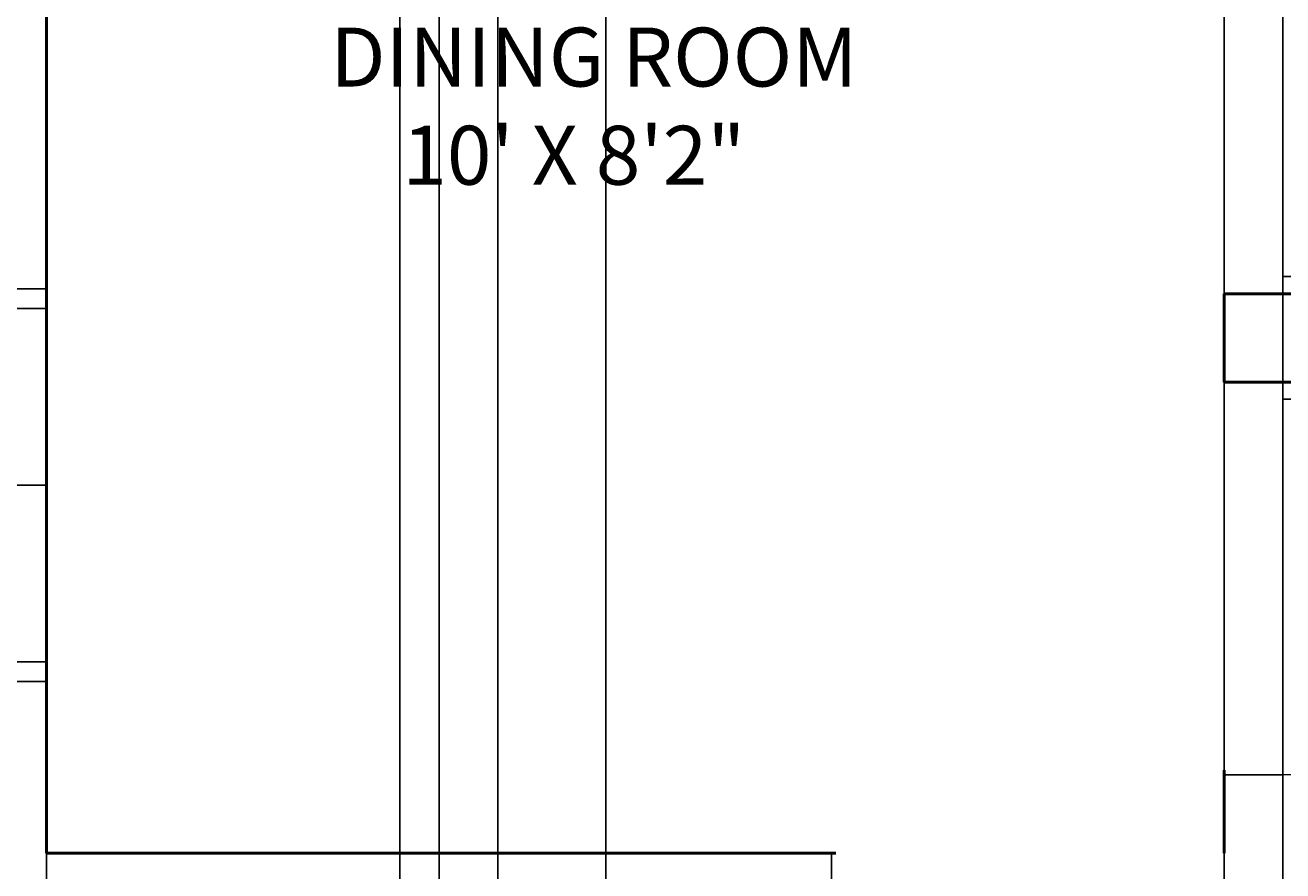
# Model space of a CAD drawing. Units: inches. Extents: x 37 to 824, y -700 to 234.
# Tile 36 of 77: x 168 to 296, y -161 to -75. Entities that reach past the tile are written whole.
import ezdxf

# ---------------------------------------------------------------- set-up
doc = ezdxf.new("R2010")
doc.units = ezdxf.units.IN
doc.header["$MEASUREMENT"] = 0
for name, color, linetype, lineweight in [('A-ANNO-DIMS', 2, 'Continuous', 18), ('A-AREA-IDEN', 3, 'Continuous', 18), ('A-DOOR', 4, 'Continuous', 25), ('A-GLAZ', 4, 'Continuous', 25), ('A-WALL', 2, 'Continuous', 50)]:
    doc.layers.add(name, color=color, linetype=linetype, lineweight=lineweight)
doc.styles.get("Standard").update_dxf_attribs({"font": 'arial.ttf'})
doc.dimstyles.get("Standard").update_dxf_attribs({"dimtxt": 0.18, "dimasz": 0.18, "dimexe": 0.18, "dimexo": 0.0625, "dimgap": 0.09, "dimtad": 0, "dimtih": 1, "dimtoh": 1, "dimdec": 1, "dimzin": 0, "dimdsep": 46, "dimlunit": 4, "dimtxsty": 'Standard', "dimcen": 0.09, "dimadec": 0, "dimazin": 0, "dimtfac": 1, "dimtdec": 1, "dimtofl": 0, "dimtmove": 0, "dimatfit": 3, "dimfxl": 1, "dimtolj": 1, "dimtzin": 0, "dimarcsym": 0})

# ---------------------------------------------------------------- blocks, each defined once
blk = doc.blocks.new('*U5')
for p, q in [((0, 0), (0, 6)), ((40, 0), (40, 6))]:
    blk.add_line(p, q)
blk.add_lwpolyline([(0, 0), (0, -40), (1.75, -40), (1.75, 0)], close=True)
blk.add_arc((0, 0), 40, 270, 0)
blk = doc.blocks.new('*U2')
for p, q in [((-40, 0), (-40, 6)), ((0, 0), (0, 6))]:
    blk.add_line(p, q)
blk.add_lwpolyline([(0, 0), (0, -40), (-1.75, -40), (-1.75, 0)], close=True)
blk.add_arc((0, 0), 40, 180, 270)
blk = doc.blocks.new('WIN-900')
for p, q in [((0, 9), (0, 0)), ((2, 9), (2, 0)), ((20, 9), (20, 0)), ((38, 9), (38, 0)), ((40, 9), (40, 0)), ((38, 5.5), (2, 5.5)), ((38, 3.5), (2, 3.5))]:
    blk.add_line(p, q)
blk = doc.blocks.new('*D77')
at = {"layer": 'A-ANNO-DIMS', "color": 0, "lineweight": -2, "ltscale": 0.5, "transparency": 16777216}
for p, q in [((227.08, 45.5), (227.08, -400.41)), ((290.08, 15.03), (290.08, -400.41)), ((227.26, -400.23), (258.25, -400.23)), ((289.9, -400.23), (258.91, -400.23))]:
    blk.add_line(p, q, dxfattribs=at)
at = {"layer": 'A-ANNO-DIMS', "color": 0, "ltscale": 0.5, "transparency": 16777216}
for points in [[(227.26, -400.2), (227.26, -400.26), (227.08, -400.23)], [(289.9, -400.2), (289.9, -400.26), (290.08, -400.23)]]:
    blk.add_solid(points, dxfattribs=at)
at = {"layer": 'Defpoints', "color": 0, "ltscale": 0.5, "transparency": 16777216}
for p in [(227.08, 45.56), (290.08, 15.09), (290.08, -400.23)]:
    blk.add_point(p, dxfattribs=at)
at = {"layer": 'A-ANNO-DIMS', "color": 0, "ltscale": 0.5, "transparency": 16777216, "insert": (258.58, -400.23), "char_height": 0.18, "attachment_point": 5}
blk.add_mtext('\\A1;5\'-3"', dxfattribs=at)
blk = doc.blocks.new('*D84')
at = {"layer": 'A-ANNO-DIMS', "color": 0, "lineweight": -2, "ltscale": 0.5, "transparency": 16777216}
for p, q in [((170.08, -265.85), (170.08, 234.17)), ((170.26, 233.99), (189.75, 233.99)), ((209.9, 233.99), (190.41, 233.99)), ((210.08, -265.85), (210.08, 234.17))]:
    blk.add_line(p, q, dxfattribs=at)
at = {"layer": 'A-ANNO-DIMS', "color": 0, "ltscale": 0.5, "transparency": 16777216}
for points in [[(170.26, 234.02), (170.26, 233.96), (170.08, 233.99)], [(209.9, 234.02), (209.9, 233.96), (210.08, 233.99)]]:
    blk.add_solid(points, dxfattribs=at)
at = {"layer": 'Defpoints', "color": 0, "ltscale": 0.5, "transparency": 16777216}
for p in [(210.08, 233.99), (170.08, -265.91), (210.08, -265.91)]:
    blk.add_point(p, dxfattribs=at)
at = {"layer": 'A-ANNO-DIMS', "color": 0, "ltscale": 0.5, "transparency": 16777216, "insert": (190.08, 233.99), "char_height": 0.18, "attachment_point": 5}
blk.add_mtext('\\A1;3\'-4"', dxfattribs=at)
blk = doc.blocks.new('*D85')
at = {"layer": 'A-ANNO-DIMS', "color": 0, "lineweight": -2, "ltscale": 0.5, "transparency": 16777216}
for p, q in [((170.08, -356.85), (170.08, 234.17)), ((170.26, 233.99), (187.75, 233.99)), ((205.9, 233.99), (188.41, 233.99)), ((206.08, -356.85), (206.08, 234.17))]:
    blk.add_line(p, q, dxfattribs=at)
at = {"layer": 'A-ANNO-DIMS', "color": 0, "ltscale": 0.5, "transparency": 16777216}
for points in [[(170.26, 234.02), (170.26, 233.96), (170.08, 233.99)], [(205.9, 234.02), (205.9, 233.96), (206.08, 233.99)]]:
    blk.add_solid(points, dxfattribs=at)
at = {"layer": 'Defpoints', "color": 0, "ltscale": 0.5, "transparency": 16777216}
for p in [(206.08, 233.99), (170.08, -356.91), (206.08, -356.91)]:
    blk.add_point(p, dxfattribs=at)
at = {"layer": 'A-ANNO-DIMS', "color": 0, "ltscale": 0.5, "transparency": 16777216, "insert": (188.08, 233.99), "char_height": 0.18, "attachment_point": 5}
blk.add_mtext('\\A1;3\'-0"', dxfattribs=at)
blk = doc.blocks.new('*D86')
at = {"layer": 'A-ANNO-DIMS', "color": 0, "lineweight": -2, "ltscale": 0.5, "transparency": 16777216}
for p, q in [((206.08, -356.85), (206.08, 234.17)), ((206.26, 233.99), (210.68, 233.99)), ((215.9, 233.99), (211.48, 233.99)), ((216.08, -356.85), (216.08, 234.17))]:
    blk.add_line(p, q, dxfattribs=at)
at = {"layer": 'A-ANNO-DIMS', "color": 0, "ltscale": 0.5, "transparency": 16777216}
for points in [[(206.26, 234.02), (206.26, 233.96), (206.08, 233.99)], [(215.9, 234.02), (215.9, 233.96), (216.08, 233.99)]]:
    blk.add_solid(points, dxfattribs=at)
at = {"layer": 'Defpoints', "color": 0, "ltscale": 0.5, "transparency": 16777216}
for p in [(216.08, 233.99), (206.08, -356.91), (216.08, -356.91)]:
    blk.add_point(p, dxfattribs=at)
at = {"layer": 'A-ANNO-DIMS', "color": 0, "ltscale": 0.5, "transparency": 16777216, "insert": (211.08, 233.99), "char_height": 0.18, "attachment_point": 5}
blk.add_mtext('\\A1;0\'-10"', dxfattribs=at)
blk = doc.blocks.new('*D87')
at = {"layer": 'A-ANNO-DIMS', "color": 0, "lineweight": -2, "ltscale": 0.5, "transparency": 16777216}
for p, q in [((216.08, -356.85), (216.08, 234.17)), ((216.26, 233.99), (255.75, 233.99)), ((295.9, 233.99), (256.41, 233.99)), ((296.08, -356.85), (296.08, 234.17))]:
    blk.add_line(p, q, dxfattribs=at)
at = {"layer": 'A-ANNO-DIMS', "color": 0, "ltscale": 0.5, "transparency": 16777216}
for points in [[(216.26, 234.02), (216.26, 233.96), (216.08, 233.99)], [(295.9, 234.02), (295.9, 233.96), (296.08, 233.99)]]:
    blk.add_solid(points, dxfattribs=at)
at = {"layer": 'Defpoints', "color": 0, "ltscale": 0.5, "transparency": 16777216}
for p in [(296.08, 233.99), (216.08, -356.91), (296.08, -356.91)]:
    blk.add_point(p, dxfattribs=at)
at = {"layer": 'A-ANNO-DIMS', "color": 0, "ltscale": 0.5, "transparency": 16777216, "insert": (256.08, 233.99), "char_height": 0.18, "attachment_point": 5}
blk.add_mtext('\\A1;6\'-8"', dxfattribs=at)

msp = doc.modelspace()

# ---------------------------------------------------------------- linework, layer by layer
at = {"layer": 'A-WALL'}
for p, q in [((170.08, -11.91), (170.08, -158.91)), ((419.08, -101.91), (290.08, -101.91)), ((290.08, -110.91), (290.08, -101.91)), ((419.08, -110.91), (290.08, -110.91)), ((290.08, -158.91), (290.08, -150.46)), ((250.53, -158.91), (170.08, -158.91))]:
    msp.add_line(p, q, dxfattribs=at)

# ---------------------------------------------------------------- block references
at = {"layer": 'A-DOOR', "rotation": 90}
for name, p in [('*U5', (296.08, -101.91)), ('*U2', (296.08, -110.91))]:
    msp.add_blockref(name, p, dxfattribs=at)
at = {"layer": 'A-DOOR'}
msp.add_blockref('*U2', (290.08, -164.91), dxfattribs=at)
at = {"layer": 'A-GLAZ', "rotation": 89.99999999999991}
msp.add_blockref('WIN-900', (170.08, -141.41), dxfattribs=at)

# ---------------------------------------------------------------- texts
at = {"layer": 'A-AREA-IDEN', "insert": (199, -74.8), "char_height": 6, "attachment_point": 1}
msp.add_mtext_dynamic_manual_height_columns('DINING ROOM\\P    10\' X 8\'2"', width=88.3217, gutter_width=1, heights=[0], dxfattribs=at)

# ---------------------------------------------------------------- dimensions: what is measured, and where the dimension line sits
at = {"layer": 'A-ANNO-DIMS', "ltscale": 0.5}
for base, p1, p2, picture, middle in [((210.08, 233.99), (170.08, -265.91), (210.08, -265.91), '*D84', (190.08, 233.99)), ((206.08, 233.99), (170.08, -356.91), (206.08, -356.91), '*D85', (188.08, 233.99)), ((216.08, 233.99), (206.08, -356.91), (216.08, -356.91), '*D86', (211.08, 233.99)), ((296.08, 233.99), (216.08, -356.91), (296.08, -356.91), '*D87', (256.08, 233.99)), ((290.08, -400.23), (227.08, 45.56), (290.08, 15.09), '*D77', (258.58, -400.23))]:
    dim = msp.add_linear_dim(base=base, p1=p1, p2=p2, dimstyle='Standard', override={"dimdec": 1, "dimlfac": 1, "dimrnd": 0, "dimzin": 1, "dimdsep": 46, "dimlunit": 4, "dimfrac": 2}, dxfattribs=at)
    dim.commit()
    dim.dimension.update_dxf_attribs({"geometry": picture, "text_midpoint": middle})

doc.saveas('drawing.dxf')
